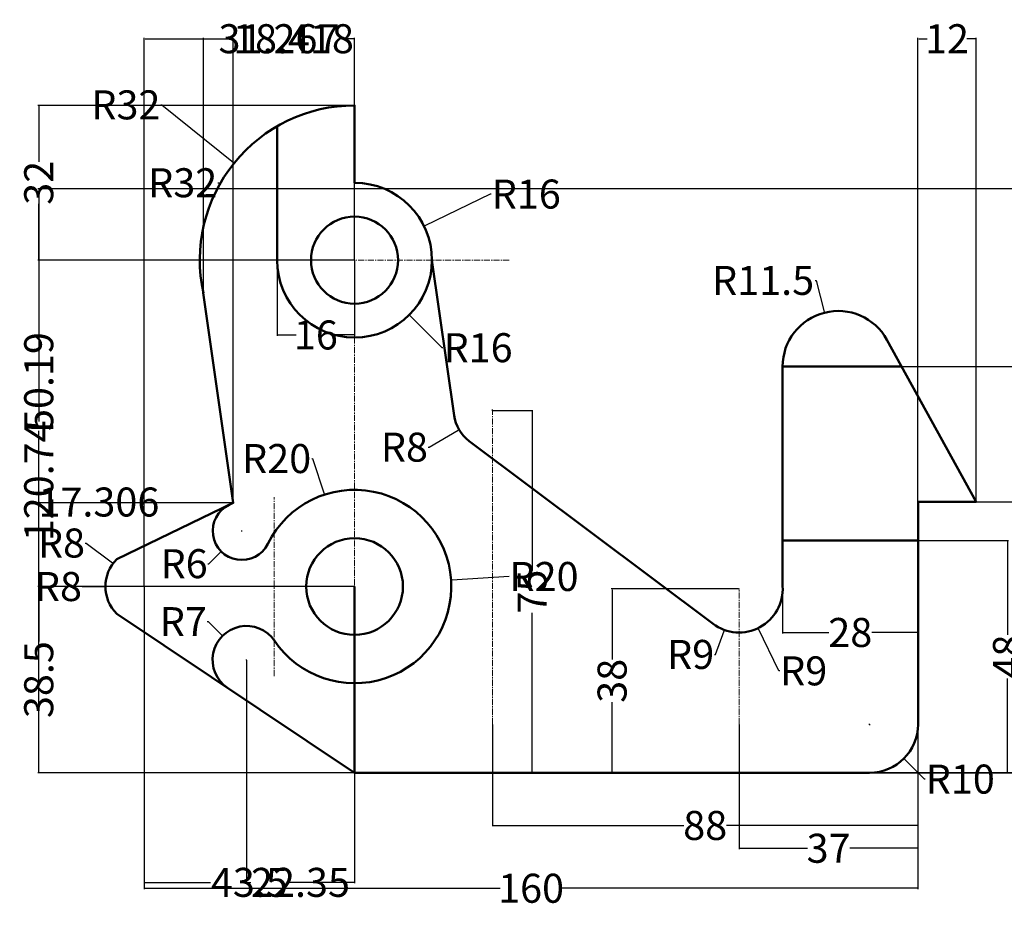
# Model space of a CAD drawing. Units: millimetres. Extents: x -1 to 307, y 9 to 193.
# Tile 1 of 2: x -1 to 203, y 9 to 193. Entities that reach past the tile are written whole.
import ezdxf

# ---------------------------------------------------------------- set-up
doc = ezdxf.new("R2010")
doc.units = ezdxf.units.MM
doc.header["$MEASUREMENT"] = 0
doc.linetypes.add('CENTER', pattern=[2, 1.25, -0.25, 0.25, -0.25])
for name, color, linetype, lineweight in [('M-CNTR', 4, 'CENTER', 18), ('M-DIMS', 2, 'Continuous', 25), ('M-OUTL', 7, 'Continuous', 50)]:
    doc.layers.add(name, color=color, linetype=linetype, lineweight=lineweight)
doc.styles.get("Standard").update_dxf_attribs({"font": 'arial.ttf'})
doc.dimstyles.get("Standard").update_dxf_attribs({"dimtxt": 6, "dimasz": 0.18, "dimexe": 0.18, "dimexo": 0.0625, "dimgap": 0.09, "dimtad": 0, "dimtoh": 1, "dimdec": 0, "dimzin": 0, "dimdsep": 46, "dimtxsty": 'Standard', "dimcen": 0.09, "dimadec": 0, "dimazin": 0, "dimtfac": 1, "dimtdec": 0, "dimtofl": 0, "dimtmove": 0, "dimatfit": 3, "dimfxl": 1, "dimtolj": 1, "dimtzin": 0, "dimarcsym": 0})

# ---------------------------------------------------------------- blocks, each defined once
blk = doc.blocks.new('*D4')
at = {"layer": 'Defpoints', "color": 0, "transparency": 16777216}
for p in [(24.86, 47.29), (184.86, 47.29), (24.86, 13.39)]:
    blk.add_point(p, dxfattribs=at)
at = {"layer": 'M-DIMS', "color": 0, "lineweight": -2, "transparency": 16777216}
for p, q in [((24.86, 47.23), (24.86, 13.21)), ((184.86, 47.23), (184.86, 13.21)), ((25.04, 13.39), (98.44, 13.39)), ((184.68, 13.39), (111.29, 13.39))]:
    blk.add_line(p, q, dxfattribs=at)
at = {"layer": 'M-DIMS', "color": 0, "transparency": 16777216}
for points in [[(25.04, 13.42), (25.04, 13.36), (24.86, 13.39)], [(184.68, 13.42), (184.68, 13.36), (184.86, 13.39)]]:
    blk.add_solid(points, dxfattribs=at)
at = {"layer": 'M-DIMS', "color": 0, "transparency": 16777216, "insert": (104.86, 13.39), "char_height": 6, "attachment_point": 5}
blk.add_mtext('\\A1;160', dxfattribs=at)
blk = doc.blocks.new('*D5')
at = {"layer": 'Defpoints', "color": 0, "transparency": 16777216}
for p in [(147.88, 47.29), (184.86, 47.29), (147.88, 21.66)]:
    blk.add_point(p, dxfattribs=at)
at = {"layer": 'M-DIMS', "color": 0, "lineweight": -2, "transparency": 16777216}
for p, q in [((147.88, 47.23), (147.88, 21.48)), ((184.86, 47.23), (184.86, 21.48)), ((148.06, 21.66), (161.99, 21.66)), ((184.68, 21.66), (170.76, 21.66))]:
    blk.add_line(p, q, dxfattribs=at)
at = {"layer": 'M-DIMS', "color": 0, "transparency": 16777216}
for points in [[(148.06, 21.69), (148.06, 21.63), (147.88, 21.66)], [(184.68, 21.69), (184.68, 21.63), (184.86, 21.66)]]:
    blk.add_solid(points, dxfattribs=at)
at = {"layer": 'M-DIMS', "color": 0, "transparency": 16777216, "insert": (166.37, 21.66), "char_height": 6, "attachment_point": 5}
blk.add_mtext('\\A1;37', dxfattribs=at)
blk = doc.blocks.new('*D6')
at = {"layer": 'Defpoints', "color": 0, "transparency": 16777216}
for p in [(96.86, 47.29), (184.86, 47.29), (96.86, 26.38)]:
    blk.add_point(p, dxfattribs=at)
at = {"layer": 'M-DIMS', "color": 0, "lineweight": -2, "transparency": 16777216}
for p, q in [((96.86, 47.23), (96.86, 26.2)), ((184.86, 47.23), (184.86, 26.2)), ((97.04, 26.38), (136.47, 26.38)), ((184.68, 26.38), (145.26, 26.38))]:
    blk.add_line(p, q, dxfattribs=at)
at = {"layer": 'M-DIMS', "color": 0, "transparency": 16777216}
for points in [[(97.04, 26.41), (97.04, 26.35), (96.86, 26.38)], [(184.68, 26.41), (184.68, 26.35), (184.86, 26.38)]]:
    blk.add_solid(points, dxfattribs=at)
at = {"layer": 'M-DIMS', "color": 0, "transparency": 16777216, "insert": (140.86, 26.38), "char_height": 6, "attachment_point": 5}
blk.add_mtext('\\A1;88', dxfattribs=at)
blk = doc.blocks.new('*D7')
at = {"layer": 'Defpoints', "color": 0, "transparency": 16777216}
for p in [(18.47, 80.59), (24.86, 75.79)]:
    blk.add_point(p, dxfattribs=at)
at = {"layer": 'M-DIMS', "color": 0, "lineweight": -2, "transparency": 16777216}
for p, q in [((12.69, 84.79), (12.87, 84.79)), ((12.87, 84.79), (18.32, 80.7)), ((24.77, 75.79), (24.95, 75.79)), ((24.86, 75.7), (24.86, 75.88))]:
    blk.add_line(p, q, dxfattribs=at)
at = {"layer": 'M-DIMS', "color": 0, "transparency": 16777216}
blk.add_solid([(18.34, 80.72), (18.3, 80.68), (18.47, 80.59)], dxfattribs=at)
at = {"layer": 'M-DIMS', "color": 0, "transparency": 16777216, "insert": (7.76, 84.79), "char_height": 6, "attachment_point": 5}
blk.add_mtext('\\A1;R8', dxfattribs=at)
blk = doc.blocks.new('*D8')
at = {"layer": 'Defpoints', "color": 0, "transparency": 16777216}
for p in [(96.86, 112.29), (89.96, 108.24)]:
    blk.add_point(p, dxfattribs=at)
at = {"layer": 'M-DIMS', "color": 0, "lineweight": -2, "transparency": 16777216}
for p, q in [((96.77, 112.29), (96.95, 112.29)), ((96.86, 112.2), (96.86, 112.38)), ((83.79, 104.62), (89.81, 108.15)), ((83.61, 104.62), (83.79, 104.62))]:
    blk.add_line(p, q, dxfattribs=at)
at = {"layer": 'M-DIMS', "color": 0, "transparency": 16777216}
blk.add_solid([(89.79, 108.18), (89.82, 108.12), (89.96, 108.24)], dxfattribs=at)
at = {"layer": 'M-DIMS', "color": 0, "transparency": 16777216, "insert": (78.67, 104.62), "char_height": 6, "attachment_point": 5}
blk.add_mtext('\\A1;R8', dxfattribs=at)
blk = doc.blocks.new('*D9')
at = {"layer": 'Defpoints', "color": 0, "transparency": 16777216}
for p in [(62.13, 94.79), (68.36, 75.79)]:
    blk.add_point(p, dxfattribs=at)
at = {"layer": 'M-DIMS', "color": 0, "lineweight": -2, "transparency": 16777216}
for p, q in [((59.5, 102.26), (59.68, 102.26)), ((59.68, 102.26), (62.07, 94.96)), ((68.27, 75.79), (68.45, 75.79)), ((68.36, 75.7), (68.36, 75.88))]:
    blk.add_line(p, q, dxfattribs=at)
at = {"layer": 'M-DIMS', "color": 0, "transparency": 16777216}
blk.add_solid([(62.1, 94.97), (62.04, 94.95), (62.13, 94.79)], dxfattribs=at)
at = {"layer": 'M-DIMS', "color": 0, "transparency": 16777216, "insert": (52.25, 102.26), "char_height": 6, "attachment_point": 5}
blk.add_mtext('\\A1;R20', dxfattribs=at)
blk = doc.blocks.new('*D10')
at = {"layer": 'Defpoints', "color": 0, "transparency": 16777216}
for p in [(96.86, 112.2), (105.06, 112.2), (96.86, 37.29)]:
    blk.add_point(p, dxfattribs=at)
at = {"layer": 'M-DIMS', "color": 0, "lineweight": -2, "transparency": 16777216}
for p, q in [((96.93, 112.2), (105.24, 112.2)), ((105.06, 112.02), (105.06, 79.13)), ((105.06, 37.47), (105.06, 70.36)), ((96.93, 37.29), (105.24, 37.29))]:
    blk.add_line(p, q, dxfattribs=at)
at = {"layer": 'M-DIMS', "color": 0, "transparency": 16777216}
for points in [[(105.03, 112.02), (105.09, 112.02), (105.06, 112.2)], [(105.03, 37.47), (105.09, 37.47), (105.06, 37.29)]]:
    blk.add_solid(points, dxfattribs=at)
at = {"layer": 'M-DIMS', "color": 0, "transparency": 16777216, "insert": (105.06, 74.74), "char_height": 6, "attachment_point": 5, "rotation": 90}
blk.add_mtext('\\A1;75', dxfattribs=at)
blk = doc.blocks.new('*D11')
at = {"layer": 'Defpoints', "color": 0, "transparency": 16777216}
for p in [(147.88, 75.29), (151.82, 67.19)]:
    blk.add_point(p, dxfattribs=at)
at = {"layer": 'M-DIMS', "color": 0, "lineweight": -2, "transparency": 16777216}
for p, q in [((147.88, 75.2), (147.88, 75.38)), ((147.79, 75.29), (147.97, 75.29)), ((156.12, 58.35), (151.89, 67.03)), ((156.3, 58.35), (156.12, 58.35))]:
    blk.add_line(p, q, dxfattribs=at)
at = {"layer": 'M-DIMS', "color": 0, "transparency": 16777216}
blk.add_solid([(151.92, 67.05), (151.87, 67.02), (151.82, 67.19)], dxfattribs=at)
at = {"layer": 'M-DIMS', "color": 0, "transparency": 16777216, "insert": (161.23, 58.35), "char_height": 6, "attachment_point": 5}
blk.add_mtext('\\A1;R9', dxfattribs=at)
blk = doc.blocks.new('*D12')
at = {"layer": 'Defpoints', "color": 0, "transparency": 16777216}
for p in [(147.79, 75.29), (121.61, 37.29), (147.79, 37.29)]:
    blk.add_point(p, dxfattribs=at)
at = {"layer": 'M-DIMS', "color": 0, "lineweight": -2, "transparency": 16777216}
for p, q in [((147.73, 75.29), (121.43, 75.29)), ((121.61, 75.11), (121.61, 60.68)), ((121.61, 37.47), (121.61, 51.9)), ((147.73, 37.29), (121.43, 37.29))]:
    blk.add_line(p, q, dxfattribs=at)
at = {"layer": 'M-DIMS', "color": 0, "transparency": 16777216}
for points in [[(121.58, 75.11), (121.64, 75.11), (121.61, 75.29)], [(121.58, 37.47), (121.64, 37.47), (121.61, 37.29)]]:
    blk.add_solid(points, dxfattribs=at)
at = {"layer": 'M-DIMS', "color": 0, "transparency": 16777216, "insert": (121.61, 56.29), "char_height": 6, "attachment_point": 5, "rotation": 90}
blk.add_mtext('\\A1;38', dxfattribs=at)
blk = doc.blocks.new('*D13')
at = {"layer": 'Defpoints', "color": 0, "transparency": 16777216}
for p in [(52.36, 143.29), (68.36, 143.29), (68.36, 127.82)]:
    blk.add_point(p, dxfattribs=at)
at = {"layer": 'M-DIMS', "color": 0, "lineweight": -2, "transparency": 16777216}
for p, q in [((52.36, 143.23), (52.36, 127.64)), ((68.36, 143.23), (68.36, 127.64)), ((52.54, 127.82), (56.26, 127.82)), ((68.18, 127.82), (64.47, 127.82))]:
    blk.add_line(p, q, dxfattribs=at)
at = {"layer": 'M-DIMS', "color": 0, "transparency": 16777216}
for points in [[(52.54, 127.85), (52.54, 127.79), (52.36, 127.82)], [(68.18, 127.85), (68.18, 127.79), (68.36, 127.82)]]:
    blk.add_solid(points, dxfattribs=at)
at = {"layer": 'M-DIMS', "color": 0, "transparency": 16777216, "insert": (60.36, 127.82), "char_height": 6, "attachment_point": 5}
blk.add_mtext('\\A1;16', dxfattribs=at)
blk = doc.blocks.new('*D14')
at = {"layer": 'Defpoints', "color": 0, "transparency": 16777216}
for p in [(40.55, 159.12), (68.36, 143.29)]:
    blk.add_point(p, dxfattribs=at)
at = {"layer": 'M-DIMS', "color": 0, "lineweight": -2, "transparency": 16777216}
for p, q in [((40.06, 159.3), (40.24, 159.3)), ((40.24, 159.3), (40.4, 159.21)), ((68.27, 143.29), (68.45, 143.29)), ((68.36, 143.2), (68.36, 143.38))]:
    blk.add_line(p, q, dxfattribs=at)
at = {"layer": 'M-DIMS', "color": 0, "transparency": 16777216}
blk.add_solid([(40.41, 159.23), (40.38, 159.18), (40.55, 159.12)], dxfattribs=at)
at = {"layer": 'M-DIMS', "color": 0, "transparency": 16777216, "insert": (32.83, 159.3), "char_height": 6, "attachment_point": 5}
blk.add_mtext('\\A1;R32', dxfattribs=at)
blk = doc.blocks.new('*D15')
at = {"layer": 'Defpoints', "color": 0, "transparency": 16777216}
for p in [(82.75, 150.3), (68.36, 143.29)]:
    blk.add_point(p, dxfattribs=at)
at = {"layer": 'M-DIMS', "color": 0, "lineweight": -2, "transparency": 16777216}
for p, q in [((96.42, 156.96), (82.91, 150.37)), ((96.6, 156.96), (96.42, 156.96)), ((68.27, 143.29), (68.45, 143.29)), ((68.36, 143.2), (68.36, 143.38))]:
    blk.add_line(p, q, dxfattribs=at)
at = {"layer": 'M-DIMS', "color": 0, "transparency": 16777216}
blk.add_solid([(82.9, 150.4), (82.92, 150.35), (82.75, 150.3)], dxfattribs=at)
at = {"layer": 'M-DIMS', "color": 0, "transparency": 16777216, "insert": (103.86, 156.96), "char_height": 6, "attachment_point": 5}
blk.add_mtext('\\A1;R16', dxfattribs=at)
blk = doc.blocks.new('*D16')
at = {"layer": 'Defpoints', "color": 0, "transparency": 16777216}
for p in [(156.86, 85.29), (184.86, 85.29), (184.86, 66.29)]:
    blk.add_point(p, dxfattribs=at)
at = {"layer": 'M-DIMS', "color": 0, "lineweight": -2, "transparency": 16777216}
for p, q in [((156.86, 85.23), (156.86, 66.11)), ((184.86, 85.23), (184.86, 66.11)), ((157.04, 66.29), (166.42, 66.29)), ((184.68, 66.29), (175.31, 66.29))]:
    blk.add_line(p, q, dxfattribs=at)
at = {"layer": 'M-DIMS', "color": 0, "transparency": 16777216}
for points in [[(157.04, 66.32), (157.04, 66.26), (156.86, 66.29)], [(184.68, 66.32), (184.68, 66.26), (184.86, 66.29)]]:
    blk.add_solid(points, dxfattribs=at)
at = {"layer": 'M-DIMS', "color": 0, "transparency": 16777216, "insert": (170.86, 66.29), "char_height": 6, "attachment_point": 5}
blk.add_mtext('\\A1;28', dxfattribs=at)
blk = doc.blocks.new('*D17')
at = {"layer": 'Defpoints', "color": 0, "transparency": 16777216}
for p in [(174.86, 85.29), (203.37, 85.29), (174.86, 37.29)]:
    blk.add_point(p, dxfattribs=at)
at = {"layer": 'M-DIMS', "color": 0, "lineweight": -2, "transparency": 16777216}
for p, q in [((174.93, 85.29), (203.55, 85.29)), ((203.37, 85.11), (203.37, 65.8)), ((203.37, 37.47), (203.37, 56.77)), ((174.93, 37.29), (203.55, 37.29))]:
    blk.add_line(p, q, dxfattribs=at)
at = {"layer": 'M-DIMS', "color": 0, "transparency": 16777216}
for points in [[(203.34, 85.11), (203.4, 85.11), (203.37, 85.29)], [(203.34, 37.47), (203.4, 37.47), (203.37, 37.29)]]:
    blk.add_solid(points, dxfattribs=at)
at = {"layer": 'M-DIMS', "color": 0, "transparency": 16777216, "insert": (203.37, 61.29), "char_height": 6, "attachment_point": 5, "rotation": 90}
blk.add_mtext('\\A1;48', dxfattribs=at)
blk = doc.blocks.new('*D18')
at = {"layer": 'Defpoints', "color": 0, "transparency": 16777216}
for p in [(190.86, 93.29), (216.03, 93.29), (174.86, 37.29)]:
    blk.add_point(p, dxfattribs=at)
at = {"layer": 'M-DIMS', "color": 0, "lineweight": -2, "transparency": 16777216}
for p, q in [((190.93, 93.29), (216.21, 93.29)), ((216.03, 93.11), (216.03, 69.67)), ((216.03, 37.47), (216.03, 60.9)), ((174.93, 37.29), (216.21, 37.29))]:
    blk.add_line(p, q, dxfattribs=at)
at = {"layer": 'M-DIMS', "color": 0, "transparency": 16777216}
for points in [[(216, 93.11), (216.06, 93.11), (216.03, 93.29)], [(216, 37.47), (216.06, 37.47), (216.03, 37.29)]]:
    blk.add_solid(points, dxfattribs=at)
at = {"layer": 'M-DIMS', "color": 0, "transparency": 16777216, "insert": (216.03, 65.29), "char_height": 6, "attachment_point": 5, "rotation": 90}
blk.add_mtext('\\A1;56', dxfattribs=at)
blk = doc.blocks.new('*D19')
at = {"layer": 'Defpoints', "color": 0, "transparency": 16777216}
for p in [(174.86, 121.29), (224.21, 121.29), (174.86, 37.29)]:
    blk.add_point(p, dxfattribs=at)
at = {"layer": 'M-DIMS', "color": 0, "lineweight": -2, "transparency": 16777216}
for p, q in [((174.93, 121.29), (224.39, 121.29)), ((224.21, 121.11), (224.21, 83.67)), ((224.21, 37.47), (224.21, 74.91)), ((174.93, 37.29), (224.39, 37.29))]:
    blk.add_line(p, q, dxfattribs=at)
at = {"layer": 'M-DIMS', "color": 0, "transparency": 16777216}
for points in [[(224.18, 121.11), (224.24, 121.11), (224.21, 121.29)], [(224.18, 37.47), (224.24, 37.47), (224.21, 37.29)]]:
    blk.add_solid(points, dxfattribs=at)
at = {"layer": 'M-DIMS', "color": 0, "transparency": 16777216, "insert": (224.21, 79.29), "char_height": 6, "attachment_point": 5, "rotation": 90}
blk.add_mtext('\\A1;84', dxfattribs=at)
blk = doc.blocks.new('*D20')
at = {"layer": 'Defpoints', "color": 0, "transparency": 16777216}
for p in [(3.06, 75.79), (68.36, 75.79), (68.36, 37.29)]:
    blk.add_point(p, dxfattribs=at)
at = {"layer": 'M-DIMS', "color": 0, "lineweight": -2, "transparency": 16777216}
for p, q in [((68.3, 75.79), (2.88, 75.79)), ((3.06, 75.61), (3.06, 64.44)), ((3.06, 37.47), (3.06, 48.64)), ((68.3, 37.29), (2.88, 37.29))]:
    blk.add_line(p, q, dxfattribs=at)
at = {"layer": 'M-DIMS', "color": 0, "transparency": 16777216}
for points in [[(3.03, 75.61), (3.09, 75.61), (3.06, 75.79)], [(3.03, 37.47), (3.09, 37.47), (3.06, 37.29)]]:
    blk.add_solid(points, dxfattribs=at)
at = {"layer": 'M-DIMS', "color": 0, "transparency": 16777216, "insert": (3.06, 56.54), "char_height": 6, "attachment_point": 5, "rotation": 90}
blk.add_mtext('\\A1;38.5', dxfattribs=at)
blk = doc.blocks.new('*D21')
at = {"layer": 'Defpoints', "color": 0, "transparency": 16777216}
for p in [(3.06, 93.09), (43.28, 93.09), (68.36, 75.79)]:
    blk.add_point(p, dxfattribs=at)
at = {"layer": 'M-DIMS', "color": 0, "lineweight": -2, "transparency": 16777216}
for p, q in [((43.22, 93.09), (2.88, 93.09)), ((3.06, 93.09), (3.06, 93.27)), ((3.06, 93.27), (3.24, 93.27)), ((3.06, 75.97), (3.06, 92.91)), ((68.3, 75.79), (2.88, 75.79))]:
    blk.add_line(p, q, dxfattribs=at)
at = {"layer": 'M-DIMS', "color": 0, "transparency": 16777216}
for points in [[(3.03, 92.91), (3.09, 92.91), (3.06, 93.09)], [(3.03, 75.97), (3.09, 75.97), (3.06, 75.79)]]:
    blk.add_solid(points, dxfattribs=at)
at = {"layer": 'M-DIMS', "color": 0, "transparency": 16777216, "insert": (15.5, 93.27), "char_height": 6, "attachment_point": 5}
blk.add_mtext('\\A1;17.306', dxfattribs=at)
blk = doc.blocks.new('*D22')
at = {"layer": 'Defpoints', "color": 0, "transparency": 16777216}
for p in [(3.06, 143.29), (68.36, 143.29), (43.28, 93.09)]:
    blk.add_point(p, dxfattribs=at)
at = {"layer": 'M-DIMS', "color": 0, "lineweight": -2, "transparency": 16777216}
for p, q in [((68.3, 143.29), (2.88, 143.29)), ((3.06, 143.11), (3.06, 128.41)), ((3.06, 93.27), (3.06, 107.97)), ((43.22, 93.09), (2.88, 93.09))]:
    blk.add_line(p, q, dxfattribs=at)
at = {"layer": 'M-DIMS', "color": 0, "transparency": 16777216}
for points in [[(3.03, 143.11), (3.09, 143.11), (3.06, 143.29)], [(3.03, 93.27), (3.09, 93.27), (3.06, 93.09)]]:
    blk.add_solid(points, dxfattribs=at)
at = {"layer": 'M-DIMS', "color": 0, "transparency": 16777216, "insert": (3.06, 118.19), "char_height": 6, "attachment_point": 5, "rotation": 90}
blk.add_mtext('\\A1;50.19', dxfattribs=at)
blk = doc.blocks.new('*D23')
at = {"layer": 'Defpoints', "color": 0, "transparency": 16777216}
for p in [(3.06, 175.29), (68.36, 175.29), (68.36, 143.29)]:
    blk.add_point(p, dxfattribs=at)
at = {"layer": 'M-DIMS', "color": 0, "lineweight": -2, "transparency": 16777216}
for p, q in [((68.3, 175.29), (2.88, 175.29)), ((3.06, 175.11), (3.06, 163.64)), ((3.06, 143.47), (3.06, 154.93)), ((68.3, 143.29), (2.88, 143.29))]:
    blk.add_line(p, q, dxfattribs=at)
at = {"layer": 'M-DIMS', "color": 0, "transparency": 16777216}
for points in [[(3.03, 175.11), (3.09, 175.11), (3.06, 175.29)], [(3.03, 143.47), (3.09, 143.47), (3.06, 143.29)]]:
    blk.add_solid(points, dxfattribs=at)
at = {"layer": 'M-DIMS', "color": 0, "transparency": 16777216, "insert": (3.06, 159.29), "char_height": 6, "attachment_point": 5, "rotation": 90}
blk.add_mtext('\\A1;32', dxfattribs=at)
blk = doc.blocks.new('*D24')
at = {"layer": 'Defpoints', "color": 0, "transparency": 16777216}
for p in [(24.86, 75.79), (68.36, 75.79), (68.36, 14.61)]:
    blk.add_point(p, dxfattribs=at)
at = {"layer": 'M-DIMS', "color": 0, "lineweight": -2, "transparency": 16777216}
for p, q in [((24.86, 75.73), (24.86, 14.43)), ((68.36, 75.73), (68.36, 14.43)), ((25.04, 14.61), (38.59, 14.61)), ((68.18, 14.61), (54.64, 14.61))]:
    blk.add_line(p, q, dxfattribs=at)
at = {"layer": 'M-DIMS', "color": 0, "transparency": 16777216}
for points in [[(25.04, 14.64), (25.04, 14.58), (24.86, 14.61)], [(68.18, 14.64), (68.18, 14.58), (68.36, 14.61)]]:
    blk.add_solid(points, dxfattribs=at)
at = {"layer": 'M-DIMS', "color": 0, "transparency": 16777216, "insert": (46.61, 14.61), "char_height": 6, "attachment_point": 5}
blk.add_mtext('\\A1;43.5', dxfattribs=at)
blk = doc.blocks.new('*D25')
at = {"layer": 'Defpoints', "color": 0, "transparency": 16777216}
for p in [(68.36, 75.79), (46.01, 60.64), (68.36, 14.61)]:
    blk.add_point(p, dxfattribs=at)
at = {"layer": 'M-DIMS', "color": 0, "lineweight": -2, "transparency": 16777216}
for p, q in [((68.36, 75.73), (68.36, 14.43)), ((46.01, 60.58), (46.01, 14.43)), ((46.19, 14.61), (46.9, 14.61)), ((68.18, 14.61), (67.47, 14.61))]:
    blk.add_line(p, q, dxfattribs=at)
at = {"layer": 'M-DIMS', "color": 0, "transparency": 16777216}
for points in [[(46.19, 14.64), (46.19, 14.58), (46.01, 14.61)], [(68.18, 14.64), (68.18, 14.58), (68.36, 14.61)]]:
    blk.add_solid(points, dxfattribs=at)
at = {"layer": 'M-DIMS', "color": 0, "transparency": 16777216, "insert": (57.19, 14.61), "char_height": 6, "attachment_point": 5}
blk.add_mtext('\\A1;22.35', dxfattribs=at)
blk = doc.blocks.new('*D26')
at = {"layer": 'Defpoints', "color": 0, "transparency": 16777216}
for p in [(43.28, 189.09), (43.28, 93.09), (24.86, 75.79)]:
    blk.add_point(p, dxfattribs=at)
at = {"layer": 'M-DIMS', "color": 0, "lineweight": -2, "transparency": 16777216}
for p, q in [((24.86, 75.85), (24.86, 189.27)), ((25.04, 189.09), (43.1, 189.09)), ((43.28, 93.16), (43.28, 189.27)), ((43.28, 189.09), (43.46, 189.09))]:
    blk.add_line(p, q, dxfattribs=at)
at = {"layer": 'M-DIMS', "color": 0, "transparency": 16777216}
for points in [[(25.04, 189.12), (25.04, 189.06), (24.86, 189.09)], [(43.1, 189.12), (43.1, 189.06), (43.28, 189.09)]]:
    blk.add_solid(points, dxfattribs=at)
at = {"layer": 'M-DIMS', "color": 0, "transparency": 16777216, "insert": (55.73, 189.09), "char_height": 6, "attachment_point": 5}
blk.add_mtext('\\A1;18.418', dxfattribs=at)
blk = doc.blocks.new('*D27')
at = {"layer": 'Defpoints', "color": 0, "transparency": 16777216}
for p in [(68.36, 189.09), (68.36, 143.29), (37.1, 136.48)]:
    blk.add_point(p, dxfattribs=at)
at = {"layer": 'M-DIMS', "color": 0, "lineweight": -2, "transparency": 16777216}
for p, q in [((37.1, 136.54), (37.1, 189.27)), ((37.28, 189.09), (40.19, 189.09)), ((68.18, 189.09), (65.27, 189.09)), ((68.36, 143.35), (68.36, 189.27))]:
    blk.add_line(p, q, dxfattribs=at)
at = {"layer": 'M-DIMS', "color": 0, "transparency": 16777216}
for points in [[(37.28, 189.12), (37.28, 189.06), (37.1, 189.09)], [(68.18, 189.12), (68.18, 189.06), (68.36, 189.09)]]:
    blk.add_solid(points, dxfattribs=at)
at = {"layer": 'M-DIMS', "color": 0, "transparency": 16777216, "insert": (52.73, 189.09), "char_height": 6, "attachment_point": 5}
blk.add_mtext('\\A1;31.267', dxfattribs=at)
blk = doc.blocks.new('*D28')
at = {"layer": 'Defpoints', "color": 0, "transparency": 16777216}
for p in [(196.86, 189.09), (184.86, 93.29), (196.86, 93.29)]:
    blk.add_point(p, dxfattribs=at)
at = {"layer": 'M-DIMS', "color": 0, "lineweight": -2, "transparency": 16777216}
for p, q in [((184.86, 93.35), (184.86, 189.27)), ((185.04, 189.09), (186.79, 189.09)), ((196.68, 189.09), (194.94, 189.09)), ((196.86, 93.35), (196.86, 189.27))]:
    blk.add_line(p, q, dxfattribs=at)
at = {"layer": 'M-DIMS', "color": 0, "transparency": 16777216}
for points in [[(185.04, 189.12), (185.04, 189.06), (184.86, 189.09)], [(196.68, 189.12), (196.68, 189.06), (196.86, 189.09)]]:
    blk.add_solid(points, dxfattribs=at)
at = {"layer": 'M-DIMS', "color": 0, "transparency": 16777216, "insert": (190.86, 189.09), "char_height": 6, "attachment_point": 5}
blk.add_mtext('\\A1;12', dxfattribs=at)
blk = doc.blocks.new('*D29')
at = {"layer": 'Defpoints', "color": 0, "transparency": 16777216}
for p in [(3.06, 158.03), (246.01, 158.03), (252.51, 37.29)]:
    blk.add_point(p, dxfattribs=at)
at = {"layer": 'M-DIMS', "color": 0, "lineweight": -2, "transparency": 16777216}
for p, q in [((245.95, 158.03), (2.88, 158.03)), ((3.06, 157.85), (3.06, 109.91)), ((3.06, 37.47), (3.06, 85.41)), ((252.45, 37.29), (2.88, 37.29))]:
    blk.add_line(p, q, dxfattribs=at)
at = {"layer": 'M-DIMS', "color": 0, "transparency": 16777216}
for points in [[(3.03, 157.85), (3.09, 157.85), (3.06, 158.03)], [(3.03, 37.47), (3.09, 37.47), (3.06, 37.29)]]:
    blk.add_solid(points, dxfattribs=at)
at = {"layer": 'M-DIMS', "color": 0, "transparency": 16777216, "insert": (3.06, 97.66), "char_height": 6, "attachment_point": 5, "rotation": 90}
blk.add_mtext('\\A1;120.74', dxfattribs=at)
blk = doc.blocks.new('*D39')
at = {"layer": 'Defpoints', "color": 0, "transparency": 16777216}
for p in [(43.44, 163.36), (68.36, 143.29)]:
    blk.add_point(p, dxfattribs=at)
at = {"layer": 'M-DIMS', "color": 0, "lineweight": -2, "transparency": 16777216}
for p, q in [((28.31, 175.41), (28.49, 175.41)), ((28.49, 175.41), (43.3, 163.48)), ((68.27, 143.29), (68.45, 143.29)), ((68.36, 143.2), (68.36, 143.38))]:
    blk.add_line(p, q, dxfattribs=at)
at = {"layer": 'M-DIMS', "color": 0, "transparency": 16777216}
blk.add_solid([(43.32, 163.5), (43.28, 163.45), (43.44, 163.36)], dxfattribs=at)
at = {"layer": 'M-DIMS', "color": 0, "transparency": 16777216, "insert": (21.08, 175.41), "char_height": 6, "attachment_point": 5}
blk.add_mtext('\\A1;R32', dxfattribs=at)
blk = doc.blocks.new('*D40')
at = {"layer": 'Defpoints', "color": 0, "transparency": 16777216}
for p in [(68.36, 143.29), (79.68, 131.97)]:
    blk.add_point(p, dxfattribs=at)
at = {"layer": 'M-DIMS', "color": 0, "lineweight": -2, "transparency": 16777216}
for p, q in [((68.27, 143.29), (68.45, 143.29)), ((68.36, 143.2), (68.36, 143.38)), ((86.46, 125.19), (79.8, 131.85)), ((86.64, 125.19), (86.46, 125.19))]:
    blk.add_line(p, q, dxfattribs=at)
at = {"layer": 'M-DIMS', "color": 0, "transparency": 16777216}
blk.add_solid([(79.82, 131.87), (79.78, 131.83), (79.68, 131.97)], dxfattribs=at)
at = {"layer": 'M-DIMS', "color": 0, "transparency": 16777216, "insert": (93.9, 125.19), "char_height": 6, "attachment_point": 5}
blk.add_mtext('\\A1;R16', dxfattribs=at)
blk = doc.blocks.new('*D41')
at = {"layer": 'Defpoints', "color": 0, "transparency": 16777216}
for p in [(68.36, 75.79), (88.32, 77.09)]:
    blk.add_point(p, dxfattribs=at)
at = {"layer": 'M-DIMS', "color": 0, "lineweight": -2, "transparency": 16777216}
for p, q in [((100.3, 77.87), (88.5, 77.1)), ((68.27, 75.79), (68.45, 75.79)), ((68.36, 75.7), (68.36, 75.88))]:
    blk.add_line(p, q, dxfattribs=at)
at = {"layer": 'M-DIMS', "color": 0, "transparency": 16777216}
blk.add_solid([(88.5, 77.13), (88.5, 77.07), (88.32, 77.09)], dxfattribs=at)
at = {"layer": 'M-DIMS', "color": 0, "transparency": 16777216, "insert": (107.54, 77.87), "char_height": 6, "attachment_point": 5}
blk.add_mtext('\\A1;R20', dxfattribs=at)
blk = doc.blocks.new('*D42')
at = {"layer": 'Defpoints', "color": 0, "transparency": 16777216}
for p in [(16.86, 75.79), (24.86, 75.79)]:
    blk.add_point(p, dxfattribs=at)
at = {"layer": 'M-DIMS', "color": 0, "lineweight": -2, "transparency": 16777216}
for p, q in [((12.06, 75.79), (16.68, 75.79)), ((24.77, 75.79), (24.95, 75.79)), ((24.86, 75.7), (24.86, 75.88))]:
    blk.add_line(p, q, dxfattribs=at)
at = {"layer": 'M-DIMS', "color": 0, "transparency": 16777216}
blk.add_solid([(16.68, 75.82), (16.68, 75.76), (16.86, 75.79)], dxfattribs=at)
at = {"layer": 'M-DIMS', "color": 0, "transparency": 16777216, "insert": (7.13, 75.79), "char_height": 6, "attachment_point": 5}
blk.add_mtext('\\A1;R8', dxfattribs=at)
blk = doc.blocks.new('*D43')
at = {"layer": 'Defpoints', "color": 0, "transparency": 16777216}
for p in [(147.88, 75.29), (144.81, 66.83)]:
    blk.add_point(p, dxfattribs=at)
at = {"layer": 'M-DIMS', "color": 0, "lineweight": -2, "transparency": 16777216}
for p, q in [((147.88, 75.2), (147.88, 75.38)), ((147.79, 75.29), (147.97, 75.29)), ((142.97, 61.75), (144.75, 66.66)), ((142.79, 61.75), (142.97, 61.75))]:
    blk.add_line(p, q, dxfattribs=at)
at = {"layer": 'M-DIMS', "color": 0, "transparency": 16777216}
blk.add_solid([(144.72, 66.67), (144.78, 66.65), (144.81, 66.83)], dxfattribs=at)
at = {"layer": 'M-DIMS', "color": 0, "transparency": 16777216, "insert": (137.85, 61.75), "char_height": 6, "attachment_point": 5}
blk.add_mtext('\\A1;R9', dxfattribs=at)
blk = doc.blocks.new('*D44')
at = {"layer": 'Defpoints', "color": 0, "transparency": 16777216}
for p in [(41.05, 65.57), (46.01, 60.64)]:
    blk.add_point(p, dxfattribs=at)
at = {"layer": 'M-DIMS', "color": 0, "lineweight": -2, "transparency": 16777216}
for p, q in [((37.89, 68.53), (38.07, 68.53)), ((38.07, 68.53), (40.92, 65.7)), ((45.92, 60.64), (46.1, 60.64)), ((46.01, 60.55), (46.01, 60.73))]:
    blk.add_line(p, q, dxfattribs=at)
at = {"layer": 'M-DIMS', "color": 0, "transparency": 16777216}
blk.add_solid([(40.94, 65.72), (40.9, 65.68), (41.05, 65.57)], dxfattribs=at)
at = {"layer": 'M-DIMS', "color": 0, "transparency": 16777216, "insert": (32.96, 68.53), "char_height": 6, "attachment_point": 5}
blk.add_mtext('\\A1;R7', dxfattribs=at)
blk = doc.blocks.new('*D45')
at = {"layer": 'Defpoints', "color": 0, "transparency": 16777216}
for p in [(45.04, 87.28), (40.78, 83.05)]:
    blk.add_point(p, dxfattribs=at)
at = {"layer": 'M-DIMS', "color": 0, "lineweight": -2, "transparency": 16777216}
for p, q in [((44.95, 87.28), (45.13, 87.28)), ((45.04, 87.19), (45.04, 87.37)), ((38.23, 80.52), (40.65, 82.93)), ((38.05, 80.52), (38.23, 80.52))]:
    blk.add_line(p, q, dxfattribs=at)
at = {"layer": 'M-DIMS', "color": 0, "transparency": 16777216}
blk.add_solid([(40.63, 82.95), (40.68, 82.9), (40.78, 83.05)], dxfattribs=at)
at = {"layer": 'M-DIMS', "color": 0, "transparency": 16777216, "insert": (33.12, 80.52), "char_height": 6, "attachment_point": 5}
blk.add_mtext('\\A1;R6', dxfattribs=at)
blk = doc.blocks.new('*D46')
at = {"layer": 'Defpoints', "color": 0, "transparency": 16777216}
for p in [(165.51, 132.43), (168.36, 121.29)]:
    blk.add_point(p, dxfattribs=at)
at = {"layer": 'M-DIMS', "color": 0, "lineweight": -2, "transparency": 16777216}
for p, q in [((163.61, 139.11), (163.79, 139.11)), ((163.79, 139.11), (165.46, 132.6)), ((168.27, 121.29), (168.45, 121.29)), ((168.36, 121.2), (168.36, 121.38))]:
    blk.add_line(p, q, dxfattribs=at)
at = {"layer": 'M-DIMS', "color": 0, "transparency": 16777216}
blk.add_solid([(165.49, 132.61), (165.43, 132.59), (165.51, 132.43)], dxfattribs=at)
at = {"layer": 'M-DIMS', "color": 0, "transparency": 16777216, "insert": (152.83, 139.11), "char_height": 6, "attachment_point": 5}
blk.add_mtext('\\A1;R11.5', dxfattribs=at)
blk = doc.blocks.new('*D47')
at = {"layer": 'Defpoints', "color": 0, "transparency": 16777216}
for p in [(174.86, 47.29), (181.93, 40.22)]:
    blk.add_point(p, dxfattribs=at)
at = {"layer": 'M-DIMS', "color": 0, "lineweight": -2, "transparency": 16777216}
for p, q in [((174.77, 47.29), (174.95, 47.29)), ((174.86, 47.2), (174.86, 47.38)), ((186.18, 35.97), (182.06, 40.09)), ((186.36, 35.97), (186.18, 35.97))]:
    blk.add_line(p, q, dxfattribs=at)
at = {"layer": 'M-DIMS', "color": 0, "transparency": 16777216}
blk.add_solid([(182.08, 40.11), (182.04, 40.07), (181.93, 40.22)], dxfattribs=at)
at = {"layer": 'M-DIMS', "color": 0, "transparency": 16777216, "insert": (193.6, 35.97), "char_height": 6, "attachment_point": 5}
blk.add_mtext('\\A1;R10', dxfattribs=at)

msp = doc.modelspace()

# ---------------------------------------------------------------- linework, layer by layer
at = {"layer": 'M-CNTR'}
for p, q in [((68.3627, 143.2884), (36.3627, 143.2884)), ((96.8627, 37.2884), (96.8627, 112.2884))]:
    msp.add_line(p, q, dxfattribs=at)
for points in [[(100.3627, 143.2884), (68.3627, 143.2884), (68.3627, 75.7884), (16.8627, 75.7884)], [(51.7192, 57.2884), (51.7192, 75.7884), (51.7192, 94.2884)], [(147.88, 28.4054), (147.88, 37.2884), (147.88, 75.2884)]]:
    msp.add_lwpolyline(points, dxfattribs=at)
at = {"layer": 'M-OUTL'}
for points in [[(52.3627, 171.0012), (52.3627, 143.2884, 2.41421356), (68.3627, 159.2884), (68.3627, 175.2884, 0.47852215), (37.0959, 136.4776)], [(156.8627, 121.2884), (156.8627, 75.8457, -0.6395952), (142.4812, 68.0875), (92.0637, 105.8876, -0.19903274), (88.9428, 111.1594), (84.3627, 143.2884)], [(68.3627, 75.7884), (68.3627, 37.2884), (19.2058, 70.1315, -0.41421356), (19.2058, 81.4452), (43.2803, 93.0941), (37.0833, 136.566)], [(181.4832, 121.2884), (156.8627, 121.2884, -0.77582982), (178.4423, 126.8247), (196.8627, 93.2884), (184.8627, 93.2884), (184.8627, 85.2884), (156.8627, 85.2884)], [(42.4268, 92.6811, 1.40127881), (50.4223, 84.6282, -3.73803765), (51.7192, 64.6981)], [(184.8627, 85.2884), (184.8627, 47.2884, -0.41421356), (174.8627, 37.2884), (68.3627, 37.2884)]]:
    msp.add_lwpolyline(points, format="xyb", dxfattribs=at)
for centre, radius in [((68.3627, 143.2884), 9), ((51.7192, 97.1774), 0), ((68.3627, 75.7884), 10)]:
    msp.add_circle(centre, radius, dxfattribs=at)
msp.add_arc((46.0129, 60.6396), 7, 34.129582, 236.251945, dxfattribs=at)

# ---------------------------------------------------------------- dimensions: what is measured, and where the dimension line sits
at = {"layer": 'M-DIMS'}
for base, p1, p2, override, picture, middle in [((43.2803, 189.0884), (24.8627, 75.7884), (43.2803, 93.0941), {"dimdec": 3, "dimlfac": 1, "dimrnd": 0, "dimzin": 0, "dimdsep": 46, "dimlunit": 2}, '*D26', (55.7283, 189.0884)), ((68.3627, 189.0884), (37.0959, 136.4776), (68.3627, 143.2884), {"dimdec": 3, "dimlfac": 1, "dimrnd": 0, "dimzin": 0, "dimdsep": 46, "dimlunit": 2}, '*D27', (52.7293, 189.0884)), ((196.8627, 189.0884), (184.8627, 93.2884), (196.8627, 93.2884), {"dimdec": 0, "dimlfac": 1, "dimrnd": 0, "dimzin": 0, "dimdsep": 46, "dimlunit": 2}, '*D28', (190.8627, 189.0884)), ((68.3627, 127.8181), (52.3627, 143.2884), (68.3627, 143.2884), {"dimclrd": 0, "dimclre": 0, "dimclrt": 0}, '*D13', (60.3627, 127.8181)), ((184.8627, 66.2884), (156.8627, 85.2884), (184.8627, 85.2884), {"dimclrd": 0, "dimclre": 0, "dimclrt": 0}, '*D16', (170.8627, 66.2884)), ((68.3627, 14.6054), (24.8627, 75.7884), (68.3627, 75.7884), {"dimdec": 1, "dimlfac": 1, "dimrnd": 0, "dimzin": 0, "dimdsep": 46, "dimlunit": 2}, '*D24', (46.6127, 14.6054)), ((68.3627, 14.6054), (46.0129, 60.6396), (68.3627, 75.7884), {"dimdec": 2, "dimlfac": 1, "dimrnd": 0, "dimzin": 0, "dimdsep": 46, "dimlunit": 2}, '*D25', (57.1878, 14.6054)), ((24.8627, 13.3864), (184.8627, 47.2884), (24.8627, 47.2884), {"dimclrd": 0, "dimclre": 0, "dimclrt": 0}, '*D4', (104.8627, 13.3864)), ((96.8627, 26.3816), (184.8627, 47.2884), (96.8627, 47.2884), {"dimclrd": 0, "dimclre": 0, "dimclrt": 0}, '*D6', (140.8627, 26.3816)), ((147.88, 21.6566), (184.8627, 47.2884), (147.88, 47.2884), {"dimclrd": 0, "dimclre": 0, "dimclrt": 0}, '*D5', (166.3713, 21.6566))]:
    dim = msp.add_linear_dim(base=base, p1=p1, p2=p2, dimstyle='Standard', override=override, dxfattribs=at)
    dim.commit()
    dim.dimension.update_dxf_attribs({"geometry": picture, "text_midpoint": middle})
for center, mpoint, override, picture, middle in [((68.3627, 143.2884), (43.4433, 163.3638), {"dimdec": 0, "dimlfac": 1, "dimrnd": 0, "dimzin": 0, "dimdsep": 46, "dimlunit": 2}, '*D39', (21.0838, 175.409)), ((68.3627, 143.2884), (82.7466, 150.2958), {"dimclrd": 0, "dimclre": 0, "dimclrt": 0}, '*D15', (103.8551, 156.9564)), ((68.3627, 143.2884), (79.6764, 131.9746), {"dimdec": 0, "dimlfac": 1, "dimrnd": 0, "dimzin": 0, "dimdsep": 46, "dimlunit": 2}, '*D40', (93.901, 125.1864)), ((168.3627, 121.2884), (165.5051, 132.4277), {"dimdec": 1, "dimlfac": 1, "dimrnd": 0, "dimzin": 0, "dimdsep": 46, "dimlunit": 2}, '*D46', (152.8343, 139.1112)), ((96.8627, 112.2884), (89.9619, 108.2413), {"dimclrd": 0, "dimclre": 0, "dimclrt": 0}, '*D8', (78.6716, 104.6189)), ((68.3627, 75.7884), (62.1259, 94.7911), {"dimclrd": 0, "dimclre": 0, "dimclrt": 0}, '*D9', (52.2468, 102.2584)), ((24.8627, 75.7884), (18.4652, 80.5917), {"dimclrd": 0, "dimclre": 0, "dimclrt": 0}, '*D7', (7.759, 84.7906)), ((45.0402, 87.2801), (40.782, 83.053), {"dimdec": 0, "dimlfac": 1, "dimrnd": 0, "dimzin": 0, "dimdsep": 46, "dimlunit": 2}, '*D45', (33.1215, 80.5168)), ((68.3627, 75.7884), (88.3205, 77.087), {"dimdec": 0, "dimlfac": 1, "dimrnd": 0, "dimzin": 0, "dimdsep": 46, "dimlunit": 2}, '*D41', (100.2952, 77.8662)), ((24.8627, 75.7884), (16.8627, 75.788), {"dimdec": 0, "dimlfac": 1, "dimrnd": 0, "dimzin": 0, "dimdsep": 46, "dimlunit": 2}, '*D42', (12.0627, 75.7878)), ((147.88, 75.2884), (144.8102, 66.8281), {"dimdec": 0, "dimlfac": 1, "dimrnd": 0, "dimzin": 0, "dimdsep": 46, "dimlunit": 2}, '*D43', (137.8545, 61.7519)), ((147.88, 75.2884), (151.8162, 67.1948), {"dimclrd": 0, "dimclre": 0, "dimclrt": 0}, '*D11', (161.23, 58.3529)), ((46.0129, 60.6396), (41.0469, 65.5731), {"dimdec": 0, "dimlfac": 1, "dimrnd": 0, "dimzin": 0, "dimdsep": 46, "dimlunit": 2}, '*D44', (32.9597, 68.5332)), ((174.8627, 47.2884), (181.9337, 40.2173), {"dimdec": 0, "dimlfac": 1, "dimrnd": 0, "dimzin": 0, "dimdsep": 46, "dimlunit": 2}, '*D47', (193.6046, 35.9746))]:
    dim = msp.add_radius_dim(center=center, mpoint=mpoint, dimstyle='Standard', override=override, dxfattribs=at)
    dim.commit()
    dim.dimension.update_dxf_attribs({"geometry": picture, "text_midpoint": middle, "dimtype": 164})
for base, p1, p2, override, picture, middle in [((3.0627, 175.2884), (68.3627, 143.2884), (68.3627, 175.2884), {"dimdec": 0, "dimlfac": 1, "dimrnd": 0, "dimzin": 0, "dimdsep": 46, "dimlunit": 2}, '*D23', (3.0627, 159.2884)), ((3.0627, 158.0275), (252.5104, 37.2884), (246.0104, 158.0275), {"dimdec": 2, "dimlfac": 1, "dimrnd": 0, "dimzin": 0, "dimdsep": 46, "dimlunit": 2}, '*D29', (3.0627, 97.6579)), ((3.0627, 143.2884), (43.2803, 93.0941), (68.3627, 143.2884), {"dimdec": 2, "dimlfac": 1, "dimrnd": 0, "dimzin": 0, "dimdsep": 46, "dimlunit": 2}, '*D22', (3.0627, 118.1912)), ((224.2119, 121.2884), (174.8627, 37.2884), (174.8627, 121.2884), {"dimclrd": 0, "dimclre": 0, "dimclrt": 0}, '*D19', (224.2119, 79.2884)), ((3.0627, 93.0941), (68.3627, 75.7884), (43.2803, 93.0941), {"dimdec": 3, "dimlfac": 1, "dimrnd": 0, "dimzin": 0, "dimdsep": 46, "dimlunit": 2}, '*D21', (15.5025, 93.2741)), ((216.0344, 93.2884), (174.8627, 37.2884), (190.8627, 93.2884), {"dimclrd": 0, "dimclre": 0, "dimclrt": 0}, '*D18', (216.0344, 65.2884)), ((203.3749, 85.2884), (174.8627, 37.2884), (174.8627, 85.2884), {"dimclrd": 0, "dimclre": 0, "dimclrt": 0}, '*D17', (203.3749, 61.2884)), ((3.0627, 75.7884), (68.3627, 37.2884), (68.3627, 75.7884), {"dimdec": 1, "dimlfac": 1, "dimrnd": 0, "dimzin": 0, "dimdsep": 46, "dimlunit": 2}, '*D20', (3.0627, 56.5384)), ((121.6127, 37.2884), (147.79, 75.2884), (147.79, 37.2884), {"dimclrd": 0, "dimclre": 0, "dimclrt": 0}, '*D12', (121.6127, 56.2884))]:
    dim = msp.add_linear_dim(base=base, p1=p1, p2=p2, angle=90, dimstyle='Standard', override=override, dxfattribs=at)
    dim.commit()
    dim.dimension.update_dxf_attribs({"geometry": picture, "text_midpoint": middle})
dim = msp.add_radius_dim(center=(68.3627, 143.2884), mpoint=(40.5528, 159.1191), dimstyle='Standard', override={"dimclrd": 0, "dimclre": 0, "dimclrt": 0}, dxfattribs=at)
dim.commit()
dim.dimension.update_dxf_attribs({"geometry": '*D14', "text_midpoint": (32.8322, 159.2972)})
dim = msp.add_aligned_dim(p1=(96.8627, 37.2884), p2=(96.8627, 112.1984), distance=-8.1965, dimstyle='Standard', override={"dimclrd": 0, "dimclre": 0, "dimclrt": 0}, dxfattribs=at)
dim.commit()
dim.dimension.update_dxf_attribs({"geometry": '*D10', "text_midpoint": (105.0592, 74.7434)})

doc.saveas('drawing.dxf')
